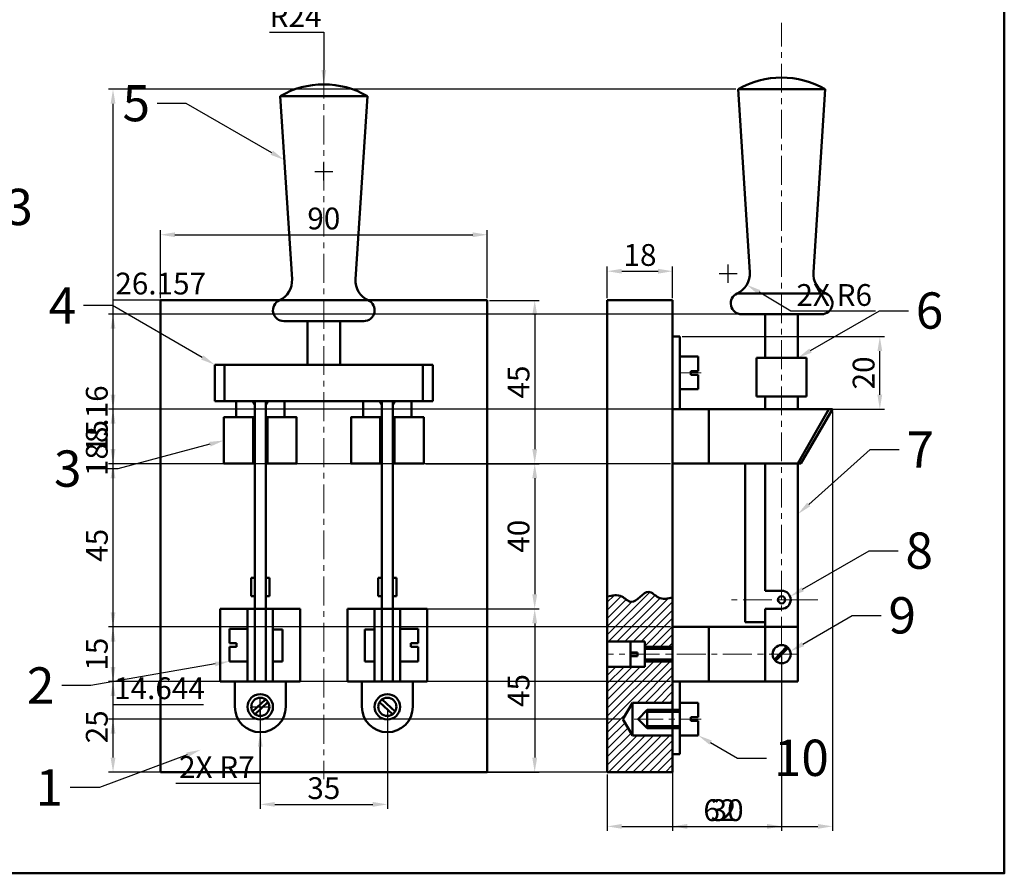
# Model space of a CAD drawing. Units: millimetres. Extents: x 1145 to 1687, y 12 to 400.
# Tile 5 of 6: x 1416 to 1687, y 12 to 247. Entities that reach past the tile are written whole.
import ezdxf
from ezdxf import colors
from ezdxf.entities.mleader import LeaderData, LeaderLine
from ezdxf.math import Vec2, Vec3

# ---------------------------------------------------------------- set-up
doc = ezdxf.new("R2010")
doc.units = ezdxf.units.MM
doc.header["$LTSCALE"] = 0.5
doc.linetypes.add('CENTER', pattern=[50.8, 31.75, -6.35, 6.35, -6.35])
for name, color, linetype, lineweight in [('M-CNTR', 1, 'CENTER', 18), ('M-DIMS', 2, 'Continuous', 25), ('M-HATC', 8, 'Continuous', 18), ('M-OUTL', 7, 'Continuous', 50), ('M-TEXT', 3, 'Continuous', 25)]:
    doc.layers.add(name, color=color, linetype=linetype, lineweight=lineweight)
doc.styles.get("Standard").update_dxf_attribs({"font": 'arial.ttf'})
doc.dimstyles.new('ISO-25', dxfattribs={"dimtxt": 6, "dimasz": 4, "dimexe": 1.25, "dimexo": 0.625, "dimtad": 1, "dimtoh": 1, "dimdec": 0, "dimtxsty": 'Standard', "dimcen": 2.5, "dimadec": 0, "dimazin": 0, "dimtfac": 1, "dimtdec": 0, "dimtofl": 0, "dimtmove": 0, "dimatfit": 3, "dimfxl": 1, "dimarcsym": 0})

# ---------------------------------------------------------------- blocks, each defined once
blk = doc.blocks.new('*D77')
at = {"layer": 'Defpoints', "color": 0, "ltscale": 0.5, "transparency": 16777216}
for p in [(1595.8, 178.16), (1577.8, 170.13), (1595.8, 170.13)]:
    blk.add_point(p, dxfattribs=at)
at = {"layer": 'M-DIMS', "color": 0, "lineweight": -2, "ltscale": 0.5, "transparency": 16777216}
for p, q in [((1577.8, 170.76), (1577.8, 179.41)), ((1595.8, 170.76), (1595.8, 179.41)), ((1581.8, 178.16), (1591.8, 178.16))]:
    blk.add_line(p, q, dxfattribs=at)
at = {"layer": 'M-DIMS', "color": 0, "ltscale": 0.5, "transparency": 16777216}
for points in [[(1581.8, 178.82), (1581.8, 177.49), (1577.8, 178.16)], [(1591.8, 178.82), (1591.8, 177.49), (1595.8, 178.16)]]:
    blk.add_solid(points, dxfattribs=at)
at = {"layer": 'M-DIMS', "color": 0, "ltscale": 0.5, "transparency": 16777216, "insert": (1586.8, 181.85), "char_height": 6, "attachment_point": 5}
blk.add_mtext('18', dxfattribs=at)
blk = doc.blocks.new('*D78')
at = {"layer": 'Defpoints', "color": 0, "ltscale": 0.5, "transparency": 16777216}
for p in [(1544.73, 188.21), (1454.73, 170.13), (1544.73, 170.13)]:
    blk.add_point(p, dxfattribs=at)
at = {"layer": 'M-DIMS', "color": 0, "lineweight": -2, "ltscale": 0.5, "transparency": 16777216}
for p, q in [((1454.73, 170.76), (1454.73, 189.46)), ((1458.73, 188.21), (1540.73, 188.21)), ((1544.73, 170.76), (1544.73, 189.46))]:
    blk.add_line(p, q, dxfattribs=at)
at = {"layer": 'M-DIMS', "color": 0, "ltscale": 0.5, "transparency": 16777216}
for points in [[(1458.73, 188.87), (1458.73, 187.54), (1454.73, 188.21)], [(1540.73, 188.87), (1540.73, 187.54), (1544.73, 188.21)]]:
    blk.add_solid(points, dxfattribs=at)
at = {"layer": 'M-DIMS', "color": 0, "ltscale": 0.5, "transparency": 16777216, "insert": (1499.73, 191.9), "char_height": 6, "attachment_point": 5}
blk.add_mtext('90', dxfattribs=at)
blk = doc.blocks.new('*D79')
at = {"layer": 'Defpoints', "color": 0, "ltscale": 0.5, "transparency": 16777216}
for p in [(1544.73, 170.13), (1527.23, 125.13), (1557.81, 125.13)]:
    blk.add_point(p, dxfattribs=at)
at = {"layer": 'M-DIMS', "color": 0, "lineweight": -2, "ltscale": 0.5, "transparency": 16777216}
for p, q in [((1545.36, 170.13), (1559.06, 170.13)), ((1557.81, 166.13), (1557.81, 129.13)), ((1527.86, 125.13), (1559.06, 125.13))]:
    blk.add_line(p, q, dxfattribs=at)
at = {"layer": 'M-DIMS', "color": 0, "ltscale": 0.5, "transparency": 16777216}
for points in [[(1557.14, 166.13), (1558.48, 166.13), (1557.81, 170.13)], [(1557.14, 129.13), (1558.48, 129.13), (1557.81, 125.13)]]:
    blk.add_solid(points, dxfattribs=at)
at = {"layer": 'M-DIMS', "color": 0, "ltscale": 0.5, "transparency": 16777216, "insert": (1554.13, 147.63), "char_height": 6, "attachment_point": 5, "rotation": 90}
blk.add_mtext('45', dxfattribs=at)
blk = doc.blocks.new('*D80')
at = {"layer": 'Defpoints', "color": 0, "ltscale": 0.5, "transparency": 16777216}
for p in [(1527.23, 125.13), (1527.23, 85.13), (1557.81, 85.13)]:
    blk.add_point(p, dxfattribs=at)
at = {"layer": 'M-DIMS', "color": 0, "lineweight": -2, "ltscale": 0.5, "transparency": 16777216}
for p, q in [((1527.86, 125.13), (1559.06, 125.13)), ((1557.81, 121.13), (1557.81, 89.13)), ((1527.86, 85.13), (1559.06, 85.13))]:
    blk.add_line(p, q, dxfattribs=at)
at = {"layer": 'M-DIMS', "color": 0, "ltscale": 0.5, "transparency": 16777216}
for points in [[(1557.14, 121.13), (1558.48, 121.13), (1557.81, 125.13)], [(1557.14, 89.13), (1558.48, 89.13), (1557.81, 85.13)]]:
    blk.add_solid(points, dxfattribs=at)
at = {"layer": 'M-DIMS', "color": 0, "ltscale": 0.5, "transparency": 16777216, "insert": (1554.12, 105.13), "char_height": 6, "attachment_point": 5, "rotation": 90}
blk.add_mtext('40', dxfattribs=at)
blk = doc.blocks.new('*D81')
at = {"layer": 'Defpoints', "color": 0, "ltscale": 0.5, "transparency": 16777216}
for p in [(1527.23, 85.13), (1527.23, 40.13), (1557.81, 40.13)]:
    blk.add_point(p, dxfattribs=at)
at = {"layer": 'M-DIMS', "color": 0, "lineweight": -2, "ltscale": 0.5, "transparency": 16777216}
for p, q in [((1527.86, 85.13), (1559.06, 85.13)), ((1557.81, 81.13), (1557.81, 44.13)), ((1527.86, 40.13), (1559.06, 40.13))]:
    blk.add_line(p, q, dxfattribs=at)
at = {"layer": 'M-DIMS', "color": 0, "ltscale": 0.5, "transparency": 16777216}
for points in [[(1557.14, 81.13), (1558.48, 81.13), (1557.81, 85.13)], [(1557.14, 44.13), (1558.48, 44.13), (1557.81, 40.13)]]:
    blk.add_solid(points, dxfattribs=at)
at = {"layer": 'M-DIMS', "color": 0, "ltscale": 0.5, "transparency": 16777216, "insert": (1554.13, 62.63), "char_height": 6, "attachment_point": 5, "rotation": 90}
blk.add_mtext('45', dxfattribs=at)
blk = doc.blocks.new('*D82')
at = {"layer": 'Defpoints', "color": 0, "ltscale": 0.5, "transparency": 16777216}
for p in [(1482.23, 58.13), (1517.23, 58.13), (1517.23, 31.26)]:
    blk.add_point(p, dxfattribs=at)
at = {"layer": 'M-DIMS', "color": 0, "lineweight": -2, "ltscale": 0.5, "transparency": 16777216}
for p, q in [((1482.23, 57.51), (1482.23, 30.01)), ((1517.23, 57.51), (1517.23, 30.01)), ((1486.23, 31.26), (1513.23, 31.26))]:
    blk.add_line(p, q, dxfattribs=at)
at = {"layer": 'M-DIMS', "color": 0, "ltscale": 0.5, "transparency": 16777216}
for points in [[(1486.23, 31.92), (1486.23, 30.59), (1482.23, 31.26)], [(1513.23, 31.92), (1513.23, 30.59), (1517.23, 31.26)]]:
    blk.add_solid(points, dxfattribs=at)
at = {"layer": 'M-DIMS', "color": 0, "ltscale": 0.5, "transparency": 16777216, "insert": (1499.73, 34.95), "char_height": 6, "attachment_point": 5}
blk.add_mtext('35', dxfattribs=at)
blk = doc.blocks.new('SCREW-HEAD')
at = {"ltscale": 0.5}
for p, q in [((0, 5), (4, 5)), ((0, 0), (0, 5)), ((4, 5), (4, 3)), ((4, 3), (5, 3)), ((5, 5), (5, 3)), ((5, 5), (9, 5)), ((9, 5), (9, 0)), ((9, 0), (0, 0))]:
    blk.add_line(p, q, dxfattribs=at)
blk = doc.blocks.new('HANDLE')
at = {"ltscale": 0.5}
for p, q in [((2, 62), (26, 62)), ((5.25, 11.58), (2, 62)), ((22.74, 11.58), (26, 62)), ((1.75, 5.73), (26.24, 5.73)), ((3, 0), (25, 0))]:
    blk.add_line(p, q, dxfattribs=at)
for centre, radius, start, end in [((14, 41.22), 24, 60, 120), ((-0.74, 11.19), 6, 294.5146, 3.6914), ((28.73, 11.19), 6, 176.3086, 245.4854), ((3, 3), 3, 114.5146, 270), ((25, 3), 3, 270, 65.4854)]:
    blk.add_arc(centre, radius, start, end, dxfattribs=at)
blk = doc.blocks.new('BRACKET')
at = {"ltscale": 0.5}
for p, q in [((15, 44), (0, 35.34)), ((15, 44), (15, 30)), ((0, 30), (0, 35.34)), ((0, 30), (0, 0)), ((15, 0), (15, 30)), ((35, 2), (15, 2)), ((35, 0), (35, 2)), ((0, 0), (15, 0)), ((15, 0), (35, 0))]:
    blk.add_line(p, q, dxfattribs=at)
blk = doc.blocks.new('TERMINAL-LUG-END')
at = {"ltscale": 0.5}
for p, q in [((0, 7), (0, 14)), ((14, 7), (14, 14))]:
    blk.add_line(p, q, dxfattribs=at)
blk.add_arc((7, 7), 7, 180, 0, dxfattribs=at)
blk = doc.blocks.new('TERMINAL-CLAMP')
at = {"ltscale": 0.5}
for p, q in [((0, 20), (0, 0)), ((0, 20), (22, 20)), ((22, 20), (22, 0)), ((0, 0), (22, 0))]:
    blk.add_line(p, q, dxfattribs=at)
blk = doc.blocks.new('*D102')
at = {"layer": 'Defpoints', "color": 0, "ltscale": 0.5, "transparency": 16777216}
for p in [(1441.68, 65.13), (1595.8, 65.13), (1595.8, 40.13)]:
    blk.add_point(p, dxfattribs=at)
at = {"layer": 'M-DIMS', "color": 0, "lineweight": -2, "ltscale": 0.5, "transparency": 16777216}
for p, q in [((1595.17, 65.13), (1440.43, 65.13)), ((1441.68, 44.13), (1441.68, 61.13)), ((1595.17, 40.13), (1440.43, 40.13))]:
    blk.add_line(p, q, dxfattribs=at)
at = {"layer": 'M-DIMS', "color": 0, "ltscale": 0.5, "transparency": 16777216}
for points in [[(1441.02, 61.13), (1442.35, 61.13), (1441.68, 65.13)], [(1441.02, 44.13), (1442.35, 44.13), (1441.68, 40.13)]]:
    blk.add_solid(points, dxfattribs=at)
at = {"layer": 'M-DIMS', "color": 0, "ltscale": 0.5, "transparency": 16777216, "insert": (1437.99, 52.63), "char_height": 6, "attachment_point": 5, "rotation": 90}
blk.add_mtext('25', dxfattribs=at)
blk = doc.blocks.new('*D103')
at = {"layer": 'Defpoints', "color": 0, "ltscale": 0.5, "transparency": 16777216}
for p in [(1441.68, 80.13), (1595.8, 80.13), (1595.8, 65.13)]:
    blk.add_point(p, dxfattribs=at)
at = {"layer": 'M-DIMS', "color": 0, "lineweight": -2, "ltscale": 0.5, "transparency": 16777216}
for p, q in [((1595.17, 80.13), (1440.43, 80.13)), ((1441.68, 69.13), (1441.68, 76.13)), ((1595.17, 65.13), (1440.43, 65.13))]:
    blk.add_line(p, q, dxfattribs=at)
at = {"layer": 'M-DIMS', "color": 0, "ltscale": 0.5, "transparency": 16777216}
for points in [[(1441.02, 76.13), (1442.35, 76.13), (1441.68, 80.13)], [(1441.02, 69.13), (1442.35, 69.13), (1441.68, 65.13)]]:
    blk.add_solid(points, dxfattribs=at)
at = {"layer": 'M-DIMS', "color": 0, "ltscale": 0.5, "transparency": 16777216, "insert": (1437.99, 72.63), "char_height": 6, "attachment_point": 5, "rotation": 90}
blk.add_mtext('15', dxfattribs=at)
blk = doc.blocks.new('*D104')
at = {"layer": 'Defpoints', "color": 0, "ltscale": 0.5, "transparency": 16777216}
for p in [(1441.68, 125.13), (1595.8, 125.13), (1595.8, 80.13)]:
    blk.add_point(p, dxfattribs=at)
at = {"layer": 'M-DIMS', "color": 0, "lineweight": -2, "ltscale": 0.5, "transparency": 16777216}
for p, q in [((1595.17, 125.13), (1440.43, 125.13)), ((1441.68, 84.13), (1441.68, 121.13)), ((1595.17, 80.13), (1440.43, 80.13))]:
    blk.add_line(p, q, dxfattribs=at)
at = {"layer": 'M-DIMS', "color": 0, "ltscale": 0.5, "transparency": 16777216}
for points in [[(1441.02, 121.13), (1442.35, 121.13), (1441.68, 125.13)], [(1441.02, 84.13), (1442.35, 84.13), (1441.68, 80.13)]]:
    blk.add_solid(points, dxfattribs=at)
at = {"layer": 'M-DIMS', "color": 0, "ltscale": 0.5, "transparency": 16777216, "insert": (1438.01, 102.63), "char_height": 6, "attachment_point": 5, "rotation": 90}
blk.add_mtext('45', dxfattribs=at)
blk = doc.blocks.new('*D105')
at = {"layer": 'Defpoints', "color": 0, "ltscale": 0.5, "transparency": 16777216}
for p in [(1441.68, 140.13), (1595.8, 140.13), (1595.8, 125.13)]:
    blk.add_point(p, dxfattribs=at)
at = {"layer": 'M-DIMS', "color": 0, "lineweight": -2, "ltscale": 0.5, "transparency": 16777216}
for p, q in [((1595.17, 140.13), (1440.43, 140.13)), ((1441.68, 129.13), (1441.68, 136.13)), ((1595.17, 125.13), (1440.43, 125.13))]:
    blk.add_line(p, q, dxfattribs=at)
at = {"layer": 'M-DIMS', "color": 0, "ltscale": 0.5, "transparency": 16777216}
for points in [[(1441.02, 136.13), (1442.35, 136.13), (1441.68, 140.13)], [(1441.02, 129.13), (1442.35, 129.13), (1441.68, 125.13)]]:
    blk.add_solid(points, dxfattribs=at)
at = {"layer": 'M-DIMS', "color": 0, "ltscale": 0.5, "transparency": 16777216, "insert": (1437.99, 132.63), "char_height": 6, "attachment_point": 5, "rotation": 90}
blk.add_mtext('15', dxfattribs=at)
blk = doc.blocks.new('*D106')
at = {"layer": 'Defpoints', "color": 0, "ltscale": 0.5, "transparency": 16777216}
for p in [(1639.8, 140.13), (1577.8, 40.13), (1639.8, 25.2)]:
    blk.add_point(p, dxfattribs=at)
at = {"layer": 'M-DIMS', "color": 0, "lineweight": -2, "ltscale": 0.5, "transparency": 16777216}
for p, q in [((1639.8, 139.51), (1639.8, 23.95)), ((1577.8, 39.51), (1577.8, 23.95)), ((1581.8, 25.2), (1635.8, 25.2))]:
    blk.add_line(p, q, dxfattribs=at)
at = {"layer": 'M-DIMS', "color": 0, "ltscale": 0.5, "transparency": 16777216}
for points in [[(1581.8, 25.86), (1581.8, 24.53), (1577.8, 25.2)], [(1635.8, 25.86), (1635.8, 24.53), (1639.8, 25.2)]]:
    blk.add_solid(points, dxfattribs=at)
at = {"layer": 'M-DIMS', "color": 0, "ltscale": 0.5, "transparency": 16777216, "insert": (1608.8, 28.89), "char_height": 6, "attachment_point": 5}
blk.add_mtext('62', dxfattribs=at)
blk = doc.blocks.new('*D107')
at = {"layer": 'Defpoints', "color": 0, "ltscale": 0.5, "transparency": 16777216}
for p in [(1441.68, 228.29), (1613.8, 228.29), (1577.8, 40.13)]:
    blk.add_point(p, dxfattribs=at)
at = {"layer": 'M-DIMS', "color": 0, "lineweight": -2, "ltscale": 0.5, "transparency": 16777216}
for p, q in [((1613.17, 228.29), (1440.43, 228.29)), ((1441.68, 44.13), (1441.68, 224.29)), ((1577.17, 40.13), (1440.43, 40.13))]:
    blk.add_line(p, q, dxfattribs=at)
at = {"layer": 'M-DIMS', "color": 0, "ltscale": 0.5, "transparency": 16777216}
for points in [[(1441.02, 224.29), (1442.35, 224.29), (1441.68, 228.29)], [(1441.02, 44.13), (1442.35, 44.13), (1441.68, 40.13)]]:
    blk.add_solid(points, dxfattribs=at)
at = {"layer": 'M-DIMS', "color": 0, "ltscale": 0.5, "transparency": 16777216, "insert": (1437.99, 134.21), "char_height": 6, "attachment_point": 5, "rotation": 90}
blk.add_mtext('188.16', dxfattribs=at)
blk = doc.blocks.new('*D108')
at = {"layer": 'Defpoints', "color": 0, "ltscale": 0.5, "transparency": 16777216}
for p in [(1595.8, 80.13), (1625.8, 72.63), (1625.8, 25.2)]:
    blk.add_point(p, dxfattribs=at)
at = {"layer": 'M-DIMS', "color": 0, "lineweight": -2, "ltscale": 0.5, "transparency": 16777216}
for p, q in [((1595.8, 79.51), (1595.8, 23.95)), ((1625.8, 72.01), (1625.8, 23.95)), ((1599.8, 25.2), (1621.8, 25.2))]:
    blk.add_line(p, q, dxfattribs=at)
at = {"layer": 'M-DIMS', "color": 0, "ltscale": 0.5, "transparency": 16777216}
for points in [[(1599.8, 25.86), (1599.8, 24.53), (1595.8, 25.2)], [(1621.8, 25.86), (1621.8, 24.53), (1625.8, 25.2)]]:
    blk.add_solid(points, dxfattribs=at)
at = {"layer": 'M-DIMS', "color": 0, "ltscale": 0.5, "transparency": 16777216, "insert": (1610.8, 28.89), "char_height": 6, "attachment_point": 5}
blk.add_mtext('30', dxfattribs=at)
blk = doc.blocks.new('*D109')
at = {"layer": 'Defpoints', "color": 0, "ltscale": 0.5, "transparency": 16777216}
for p in [(1441.68, 54.78), (1582.11, 54.78), (1577.8, 40.13)]:
    blk.add_point(p, dxfattribs=at)
at = {"layer": 'M-DIMS', "color": 0, "lineweight": -2, "ltscale": 0.5, "transparency": 16777216}
for p, q in [((1441.68, 54.78), (1441.68, 58.78)), ((1441.68, 58.78), (1466.63, 58.78)), ((1581.48, 54.78), (1440.43, 54.78)), ((1441.68, 44.13), (1441.68, 50.78)), ((1577.17, 40.13), (1440.43, 40.13))]:
    blk.add_line(p, q, dxfattribs=at)
at = {"layer": 'M-DIMS', "color": 0, "ltscale": 0.5, "transparency": 16777216}
for points in [[(1441.02, 50.78), (1442.35, 50.78), (1441.68, 54.78)], [(1441.02, 44.13), (1442.35, 44.13), (1441.68, 40.13)]]:
    blk.add_solid(points, dxfattribs=at)
at = {"layer": 'M-DIMS', "color": 0, "ltscale": 0.5, "transparency": 16777216, "insert": (1454.47, 62.47), "char_height": 6, "attachment_point": 5}
blk.add_mtext('14.644', dxfattribs=at)
blk = doc.blocks.new('*D110')
at = {"layer": 'Defpoints', "color": 0, "ltscale": 0.5, "transparency": 16777216}
for p in [(1441.68, 166.29), (1614.8, 166.29), (1621.3, 140.13)]:
    blk.add_point(p, dxfattribs=at)
at = {"layer": 'M-DIMS', "color": 0, "lineweight": -2, "ltscale": 0.5, "transparency": 16777216}
for p, q in [((1441.68, 166.29), (1441.68, 170.29)), ((1441.68, 170.29), (1467.32, 170.29)), ((1614.17, 166.29), (1440.43, 166.29)), ((1441.68, 144.13), (1441.68, 162.29)), ((1620.67, 140.13), (1440.43, 140.13))]:
    blk.add_line(p, q, dxfattribs=at)
at = {"layer": 'M-DIMS', "color": 0, "ltscale": 0.5, "transparency": 16777216}
for points in [[(1441.02, 162.29), (1442.35, 162.29), (1441.68, 166.29)], [(1441.02, 144.13), (1442.35, 144.13), (1441.68, 140.13)]]:
    blk.add_solid(points, dxfattribs=at)
at = {"layer": 'M-DIMS', "color": 0, "ltscale": 0.5, "transparency": 16777216, "insert": (1454.81, 173.98), "char_height": 6, "attachment_point": 5}
blk.add_mtext('26.157', dxfattribs=at)
blk = doc.blocks.new('*D111')
at = {"layer": 'Defpoints', "color": 0, "ltscale": 0.5, "transparency": 16777216}
for p in [(1597.8, 160.13), (1652.85, 160.13), (1595.8, 140.13)]:
    blk.add_point(p, dxfattribs=at)
at = {"layer": 'M-DIMS', "color": 0, "lineweight": -2, "ltscale": 0.5, "transparency": 16777216}
for p, q in [((1598.42, 160.13), (1654.1, 160.13)), ((1652.85, 144.13), (1652.85, 156.13)), ((1596.42, 140.13), (1654.1, 140.13))]:
    blk.add_line(p, q, dxfattribs=at)
at = {"layer": 'M-DIMS', "color": 0, "ltscale": 0.5, "transparency": 16777216}
for points in [[(1652.18, 156.13), (1653.51, 156.13), (1652.85, 160.13)], [(1652.18, 144.13), (1653.51, 144.13), (1652.85, 140.13)]]:
    blk.add_solid(points, dxfattribs=at)
at = {"layer": 'M-DIMS', "color": 0, "ltscale": 0.5, "transparency": 16777216, "insert": (1649.16, 150.13), "char_height": 6, "attachment_point": 5, "rotation": 90}
blk.add_mtext('20', dxfattribs=at)
blk = doc.blocks.new('*D119')
at = {"layer": 'Defpoints', "color": 0, "ltscale": 0.5, "transparency": 16777216}
for p in [(1499.73, 229.62), (1499.73, 205.62)]:
    blk.add_point(p, dxfattribs=at)
at = {"layer": 'M-DIMS', "color": 0, "lineweight": -2, "ltscale": 0.5, "transparency": 16777216}
for p, q in [((1484.79, 244.02), (1499.73, 244.02)), ((1499.73, 244.02), (1499.73, 233.62)), ((1499.73, 203.12), (1499.73, 208.12)), ((1497.23, 205.62), (1502.23, 205.62))]:
    blk.add_line(p, q, dxfattribs=at)
at = {"layer": 'M-DIMS', "color": 0, "ltscale": 0.5, "transparency": 16777216}
blk.add_solid([(1500.4, 233.62), (1499.07, 233.62), (1499.73, 229.62)], dxfattribs=at)
at = {"layer": 'M-DIMS', "color": 0, "ltscale": 0.5, "transparency": 16777216, "insert": (1491.95, 247.66), "char_height": 6, "attachment_point": 5}
blk.add_mtext('R24', dxfattribs=at)
blk = doc.blocks.new('*D120')
at = {"layer": 'Defpoints', "color": 0, "ltscale": 0.5, "transparency": 16777216}
for p in [(1482.23, 58.13), (1482.23, 51.13)]:
    blk.add_point(p, dxfattribs=at)
at = {"layer": 'M-DIMS', "color": 0, "lineweight": -2, "ltscale": 0.5, "transparency": 16777216}
for p, q in [((1482.23, 55.63), (1482.23, 60.63)), ((1479.73, 58.13), (1484.73, 58.13)), ((1482.23, 37.11), (1482.23, 47.13)), ((1458.94, 37.11), (1482.23, 37.11))]:
    blk.add_line(p, q, dxfattribs=at)
at = {"layer": 'M-DIMS', "color": 0, "ltscale": 0.5, "transparency": 16777216}
blk.add_solid([(1481.57, 47.13), (1482.9, 47.13), (1482.23, 51.13)], dxfattribs=at)
at = {"layer": 'M-DIMS', "color": 0, "ltscale": 0.5, "transparency": 16777216, "insert": (1470.27, 40.75), "char_height": 6, "attachment_point": 5}
blk.add_mtext('2X R7', dxfattribs=at)
blk = doc.blocks.new('*D121')
at = {"layer": 'Defpoints', "color": 0, "ltscale": 0.5, "transparency": 16777216}
for p in [(1611.06, 177.48), (1616.21, 174.4)]:
    blk.add_point(p, dxfattribs=at)
at = {"layer": 'M-DIMS', "color": 0, "lineweight": -2, "ltscale": 0.5, "transparency": 16777216}
for p, q in [((1611.06, 174.98), (1611.06, 179.98)), ((1608.56, 177.48), (1613.56, 177.48)), ((1628.33, 167.14), (1619.64, 172.34)), ((1651.63, 167.14), (1628.33, 167.14))]:
    blk.add_line(p, q, dxfattribs=at)
at = {"layer": 'M-DIMS', "color": 0, "ltscale": 0.5, "transparency": 16777216}
blk.add_solid([(1619.99, 172.92), (1619.3, 171.77), (1616.21, 174.4)], dxfattribs=at)
at = {"layer": 'M-DIMS', "color": 0, "ltscale": 0.5, "transparency": 16777216, "insert": (1640.29, 170.83), "char_height": 6, "attachment_point": 5}
blk.add_mtext('2X R6', dxfattribs=at)

msp = doc.modelspace()

# ---------------------------------------------------------------- hatches: boundary and pattern name
at = {"layer": 'M-HATC', "ltscale": 0.5}
h = msp.add_hatch(dxfattribs=at)
h.set_pattern_fill('ANSI31', color=256, scale=0.5)
h.set_pattern_definition([(45, (-479.3516, -223.5055), (-1.122532, 1.122532), [])])
edge = h.paths.add_edge_path()
edge.add_spline(control_points=[(1595.7981, 88.2598), (1594.455, 87.9688), (1592.0336, 87.444), (1588.5719, 91.6057), (1585.0835, 85.2802), (1581.6129, 89.3599), (1579.1872, 88.8247), (1577.7981, 88.5182)], knot_values=[0, 0, 0, 0, 3.87631709, 6.98846601, 12.57224805, 15.56070469, 19.56541111, 19.56541111, 19.56541111, 19.56541111], degree=3, periodic=0)
edge.add_line((1577.7981, 88.5182), (1577.7981, 76.1345))
edge.add_line((1577.7981, 76.1345), (1584.1572, 76.1345))
edge.add_line((1584.1572, 76.1345), (1588.1572, 76.1345))
edge.add_line((1588.1572, 76.1345), (1588.1572, 74.6345))
edge.add_line((1588.1572, 74.6345), (1595.7981, 74.6345))
edge.add_line((1595.7981, 74.6345), (1595.7981, 88.2598))
h.paths.add_polyline_path([(1588.1572, 69.1345), (1584.1572, 69.1345), (1577.7981, 69.1345), (1577.7981, 40.1345), (1595.7981, 40.1345), (1595.7981, 50.2788), (1584.7044, 50.2788), (1582.1063, 54.7788), (1584.7044, 59.2788), (1595.7981, 59.2788), (1595.7981, 70.6345), (1588.1572, 70.6345)])

# ---------------------------------------------------------------- linework, layer by layer
at = {"layer": 'M-CNTR', "ltscale": 0.5}
for p, q in [((1625.7981, 49.5797), (1625.7981, 246.6222)), ((1499.732, 233.7126), (1499.732, 38.2483)), ((1597.7981, 150.1345), (1603.6641, 150.1345)), ((1635.8068, 87.6345), (1611.1084, 87.6345)), ((1624.7981, 87.6345), (1629.3905, 87.6345)), ((1630.2981, 72.6345), (1577.7981, 72.6345)), ((1585.2422, 54.7788), (1603.6641, 54.7788))]:
    msp.add_line(p, q, dxfattribs=at)
at = {"layer": 'M-OUTL', "ltscale": 0.5}
for p, q in [((1611.7981, 172.2911), (1611.7981, 172.2911)), ((1544.732, 170.1345), (1454.732, 170.1345)), ((1454.732, 170.1345), (1454.732, 40.1345)), ((1485.732, 170.4049), (1485.732, 170.4049)), ((1544.732, 40.1345), (1544.732, 170.1345)), ((1577.7981, 170.1345), (1577.7981, 40.1345)), ((1595.7981, 170.1345), (1577.7981, 170.1345)), ((1595.7981, 40.1345), (1595.7981, 170.1345)), ((1621.2981, 166.2911), (1621.2981, 154.274)), ((1621.2981, 166.2911), (1630.2981, 166.2911)), ((1621.2981, 166.2911), (1630.2981, 166.2911)), ((1630.2981, 154.274), (1630.2981, 166.2911)), ((1495.232, 164.4049), (1495.232, 152.3878)), ((1495.232, 164.4049), (1504.232, 164.4049)), ((1495.232, 164.4049), (1504.232, 164.4049)), ((1504.232, 152.3878), (1504.232, 164.4049)), ((1499.732, 152.3878), (1469.732, 152.3878)), ((1469.732, 152.3878), (1469.732, 142.3878)), ((1472.422, 152.3878), (1472.422, 142.3878)), ((1504.232, 152.3878), (1495.232, 152.3878)), ((1529.732, 152.3878), (1504.232, 152.3878)), ((1527.042, 152.3878), (1527.042, 142.3878)), ((1529.732, 142.3878), (1529.732, 152.3878)), ((1630.2981, 154.274), (1618.907, 154.274)), ((1618.907, 154.274), (1618.907, 143.6345)), ((1630.2981, 154.274), (1632.6892, 154.274)), ((1632.6892, 154.274), (1632.6892, 143.6345)), ((1469.732, 142.3878), (1529.732, 142.3878)), ((1475.5773, 142.3878), (1475.5773, 137.9178)), ((1480.1771, 142.3878), (1480.732, 141.4746)), ((1480.732, 142.3878), (1480.732, 65.1345)), ((1483.732, 142.3878), (1483.732, 65.1345)), ((1484.2869, 142.3878), (1483.732, 141.4746)), ((1488.8867, 142.3878), (1488.8867, 137.9178)), ((1510.5773, 142.3878), (1510.5773, 137.9178)), ((1515.1771, 142.3878), (1515.732, 141.4746)), ((1515.732, 142.3878), (1515.732, 65.1345)), ((1518.732, 142.3878), (1518.732, 65.1345)), ((1519.2869, 142.3878), (1518.732, 141.4746)), ((1523.8867, 142.3878), (1523.8867, 137.9178)), ((1618.907, 143.6345), (1622.7981, 143.6345)), ((1621.2981, 140.1345), (1621.2981, 143.6345)), ((1622.7981, 143.6345), (1628.7981, 143.6345)), ((1632.6892, 143.6345), (1628.7981, 143.6345)), ((1630.2981, 140.1345), (1630.2981, 143.6345)), ((1605.7981, 125.1345), (1605.7981, 140.1345)), ((1638.832, 140.1345), (1630.2981, 125.1345)), ((1480.232, 137.9178), (1480.232, 125.1345)), ((1484.232, 137.9178), (1484.232, 125.1345)), ((1515.232, 137.9178), (1515.232, 125.1345)), ((1519.232, 137.9178), (1519.232, 125.1345)), ((1615.7981, 81.4343), (1615.7981, 125.1345)), ((1621.2981, 90.1345), (1621.2981, 125.1345)), ((1630.2981, 65.1345), (1630.2981, 125.1345)), ((1479.732, 88.6345), (1479.7244, 93.6345)), ((1479.7244, 93.6345), (1480.7244, 93.6345)), ((1484.7397, 93.6345), (1483.7397, 93.6345)), ((1484.732, 88.6345), (1484.7397, 93.6345)), ((1514.732, 88.6345), (1514.7244, 93.6345)), ((1514.7244, 93.6345), (1515.7244, 93.6345)), ((1519.7397, 93.6345), (1518.7397, 93.6345)), ((1519.732, 88.6345), (1519.7397, 93.6345)), ((1625.7981, 90.1345), (1621.2981, 90.1345)), ((1480.732, 88.6345), (1479.732, 88.6345)), ((1483.732, 88.6345), (1484.732, 88.6345)), ((1515.732, 88.6345), (1514.732, 88.6345)), ((1518.732, 88.6345), (1519.732, 88.6345)), ((1478.732, 85.1345), (1478.732, 65.1345)), ((1480.732, 85.1345), (1480.732, 65.1345)), ((1483.732, 85.1345), (1483.732, 65.1345)), ((1485.732, 85.1345), (1485.732, 65.1345)), ((1513.732, 85.1345), (1513.732, 65.1345)), ((1515.732, 85.1345), (1515.732, 65.1345)), ((1518.732, 85.1345), (1518.732, 65.1345)), ((1520.732, 85.1345), (1520.732, 65.1345)), ((1621.2981, 65.1345), (1621.2981, 85.1345)), ((1625.7981, 85.1345), (1621.2981, 85.1345)), ((1615.7981, 81.4343), (1621.2981, 81.4343)), ((1485.732, 79.4766), (1488.3976, 79.4766)), ((1488.3976, 79.4766), (1488.3976, 70.6345)), ((1513.732, 79.4766), (1511.0665, 79.4766)), ((1511.0665, 79.4766), (1511.0665, 70.6345)), ((1595.7981, 80.1345), (1595.7981, 65.1345)), ((1625.7981, 80.1345), (1595.7981, 80.1345)), ((1605.7981, 80.1345), (1605.7981, 65.1345)), ((1625.7981, 80.1345), (1630.2981, 80.1345)), ((1584.1572, 76.1345), (1577.7981, 76.1345)), ((1584.1572, 76.1345), (1584.1572, 69.1345)), ((1588.1572, 76.1345), (1584.1572, 76.1345)), ((1588.1572, 69.1345), (1588.1572, 76.1345)), ((1588.1572, 74.6345), (1595.7981, 74.6345)), ((1588.1572, 74.1345), (1595.7981, 74.1345)), ((1627.2281, 74.7247), (1623.7701, 71.1174)), ((1627.5891, 74.3787), (1624.1311, 70.7714)), ((1488.3976, 70.6345), (1485.732, 70.6345)), ((1511.0665, 70.6345), (1513.732, 70.6345)), ((1584.1572, 73.1345), (1586.1572, 73.1345)), ((1586.1572, 72.1345), (1584.1572, 72.1345)), ((1586.1572, 73.1345), (1586.1572, 72.1345)), ((1588.1572, 71.1345), (1595.7981, 71.1345)), ((1588.1572, 70.6345), (1595.7981, 70.6345)), ((1584.1572, 69.1345), (1577.7981, 69.1345)), ((1584.1572, 69.1345), (1588.1572, 69.1345)), ((1595.7981, 65.1345), (1625.7981, 65.1345)), ((1595.7981, 65.1345), (1595.7981, 45.1345)), ((1597.7981, 45.1345), (1597.7981, 65.1345)), ((1630.2981, 65.1345), (1621.2981, 65.1345)), ((1483.6776, 60.1742), (1480.1027, 56.8245)), ((1515.7865, 60.1742), (1519.3613, 56.8245)), ((1484.3613, 59.4445), (1480.7865, 56.0948)), ((1515.1027, 59.4445), (1518.6776, 56.0948)), ((1584.7044, 59.2788), (1582.1063, 54.7788)), ((1584.7044, 59.2788), (1584.7044, 50.2788)), ((1584.7044, 59.2788), (1595.7981, 59.2788)), ((1588.7981, 57.2788), (1586.2996, 54.7788)), ((1597.7981, 57.2788), (1588.7981, 57.2788)), ((1588.7981, 52.2788), (1588.7981, 57.2788)), ((1584.7044, 50.2788), (1582.1063, 54.7788)), ((1588.7981, 52.2788), (1586.2996, 54.7788)), ((1597.7981, 56.7788), (1588.7981, 56.7788)), ((1597.7981, 52.7788), (1588.7981, 52.7788)), ((1597.7981, 52.2788), (1588.7981, 52.2788)), ((1584.7044, 50.2788), (1595.7981, 50.2788)), ((1595.7981, 45.1345), (1597.7981, 45.1345)), ((1454.732, 40.1345), (1544.732, 40.1345)), ((1577.7981, 40.1345), (1595.7981, 40.1345))]:
    msp.add_line(p, q, dxfattribs=at)
msp.add_lwpolyline([(1145.3327, 400.1417), (1687.1285, 400.1417), (1687.1285, 12.2645), (1145.3327, 12.2645)], close=True, dxfattribs=at)
for points in [[(1480.732, 125.1345), (1472.232, 125.1345), (1472.232, 137.9178), (1480.732, 137.9178)], [(1483.732, 137.9178), (1492.232, 137.9178), (1492.232, 125.1345), (1483.732, 125.1345)], [(1515.732, 137.9178), (1507.232, 137.9178), (1507.232, 125.1345), (1515.732, 125.1345)], [(1518.732, 125.1345), (1527.232, 125.1345), (1527.232, 137.9178), (1518.732, 137.9178)]]:
    msp.add_lwpolyline(points, dxfattribs=at)
for centre, radius in [((1625.7981, 87.6345), 1), ((1625.7981, 87.6345), 1), ((1625.7981, 72.6345), 2.5), ((1625.7981, 72.6345), 2.5), ((1482.232, 58.1345), 3.5), ((1482.232, 58.1345), 2.5), ((1517.232, 58.1345), 3.5), ((1517.232, 58.1345), 2.5)]:
    msp.add_circle(centre, radius, dxfattribs=at)
msp.add_arc((1625.7981, 87.6345), 2.5, 270, 90, dxfattribs=at)
msp.add_open_spline([(1577.7981, 88.5182), (1579.1872, 88.8247), (1581.6129, 89.3599), (1585.0835, 85.2802), (1588.5719, 91.6057), (1592.0336, 87.444), (1594.455, 87.9688), (1595.7981, 88.2598)], degree=3, knots=[0, 0, 0, 0, 4.00470642, 6.99316306, 12.5769451, 15.68909402, 19.56541111, 19.56541111, 19.56541111, 19.56541111], dxfattribs=at)

# ---------------------------------------------------------------- block references
at = {"layer": 'M-OUTL'}
for name, p in [('HANDLE', (1485.7339, 164.4048)), ('HANDLE', (1611.8, 166.291)), ('TERMINAL-CLAMP', (1471.232, 65.134)), ('TERMINAL-CLAMP', (1506.232, 65.134)), ('TERMINAL-LUG-END', (1475.2324, 51.1344)), ('TERMINAL-LUG-END', (1510.2324, 51.1344))]:
    msp.add_blockref(name, p, dxfattribs=at)
at = {"layer": 'M-OUTL', "extrusion": (0, 0, -1), "zscale": -1, "rotation": 89.99999999999916}
msp.add_blockref('BRACKET', (-1595.7984, 125.1344), dxfattribs=at)
at = {"layer": 'M-OUTL'}
for p, rotation in [((1597.7983, 154.6349), 269.9999999999989), ((1478.7318, 70.634), 90.0000000000044), ((1520.7323, 79.6349), 269.9999999999964), ((1597.7983, 59.2792), 269.9999999999986)]:
    msp.add_blockref('SCREW-HEAD', p, dxfattribs=dict(at, rotation=rotation))

# ---------------------------------------------------------------- dimensions: what is measured, and where the dimension line sits
at = {"layer": 'M-DIMS', "ltscale": 0.5}
dim = msp.add_radius_dim(center=(1499.732, 205.6203), mpoint=(1499.732, 229.6203), dimstyle='ISO-25', override={"dimdec": 0, "dimlfac": 1, "dimrnd": 0, "dimzin": 0, "dimdsep": 46, "dimlunit": 2}, dxfattribs=at)
dim.commit()
dim.dimension.update_dxf_attribs({"geometry": '*D119', "text_midpoint": (1491.9508, 244.0203), "dimtype": 164})
for base, p1, p2, override, picture, middle in [((1441.682, 228.2911), (1577.7981, 40.1345), (1613.7981, 228.2911), {"dimdec": 2, "dimlfac": 1, "dimrnd": 0, "dimzin": 0, "dimdsep": 46, "dimlunit": 2}, '*D107', (1437.9936, 134.2128)), ((1441.682, 166.2911), (1621.2981, 140.1345), (1614.7981, 166.2911), {"dimdec": 3, "dimlfac": 1, "dimrnd": 0, "dimzin": 0, "dimdsep": 46, "dimlunit": 2}, '*D110', (1454.8125, 173.9795)), ((1557.811, 125.1345), (1544.732, 170.1345), (1527.232, 125.1345), {"dimclrd": 0, "dimclre": 0, "dimclrt": 0}, '*D79', (1554.1348, 147.6345)), ((1652.8481, 160.1345), (1595.7981, 140.1345), (1597.7981, 160.1345), {"dimdec": 0, "dimlfac": 1, "dimrnd": 0, "dimzin": 0, "dimdsep": 46, "dimlunit": 2}, '*D111', (1649.1596, 150.1345)), ((1441.682, 140.1345), (1595.7981, 125.1345), (1595.7981, 140.1345), {"dimdec": 0, "dimlfac": 1, "dimrnd": 0, "dimzin": 0, "dimdsep": 46, "dimlunit": 2}, '*D105', (1437.9936, 132.6345)), ((1441.682, 125.1345), (1595.7981, 80.1345), (1595.7981, 125.1345), {"dimdec": 0, "dimlfac": 1, "dimrnd": 0, "dimzin": 0, "dimdsep": 46, "dimlunit": 2}, '*D104', (1438.0059, 102.6345)), ((1557.811, 85.1345), (1527.232, 125.1345), (1527.232, 85.1345), {"dimclrd": 0, "dimclre": 0, "dimclrt": 0}, '*D80', (1554.1225, 105.1345)), ((1557.811, 40.1345), (1527.232, 85.1345), (1527.232, 40.1345), {"dimclrd": 0, "dimclre": 0, "dimclrt": 0}, '*D81', (1554.1348, 62.6345)), ((1441.682, 80.1345), (1595.7981, 65.1345), (1595.7981, 80.1345), {"dimdec": 0, "dimlfac": 1, "dimrnd": 0, "dimzin": 0, "dimdsep": 46, "dimlunit": 2}, '*D103', (1437.9936, 72.6345)), ((1441.682, 65.1345), (1595.7981, 40.1345), (1595.7981, 65.1345), {"dimdec": 0, "dimlfac": 1, "dimrnd": 0, "dimzin": 0, "dimdsep": 46, "dimlunit": 2}, '*D102', (1437.9936, 52.6345)), ((1441.682, 54.7788), (1577.7981, 40.1345), (1582.1063, 54.7788), {"dimdec": 3, "dimlfac": 1, "dimrnd": 0, "dimzin": 0, "dimdsep": 46, "dimlunit": 2}, '*D109', (1454.4666, 62.4672))]:
    dim = msp.add_linear_dim(base=base, p1=p1, p2=p2, angle=90, dimstyle='ISO-25', override=override, dxfattribs=at)
    dim.commit()
    dim.dimension.update_dxf_attribs({"geometry": picture, "text_midpoint": middle})
for base, p1, p2, override, picture, middle in [((1544.732, 188.2072), (1454.732, 170.1345), (1544.732, 170.1345), {"dimclrd": 0, "dimclre": 0, "dimclrt": 0}, '*D78', (1499.732, 191.8957)), ((1595.7981, 178.1569), (1577.7981, 170.1345), (1595.7981, 170.1345), {"dimclrd": 0, "dimclre": 0, "dimclrt": 0}, '*D77', (1586.7981, 181.8454)), ((1639.7981, 25.1983), (1577.7981, 40.1345), (1639.7981, 140.1345), {"dimdec": 0, "dimlfac": 1, "dimrnd": 0, "dimzin": 0, "dimdsep": 46, "dimlunit": 2}, '*D106', (1608.7981, 28.8867)), ((1625.7981, 25.1983), (1595.7981, 80.1345), (1625.7981, 72.6345), {"dimdec": 0, "dimlfac": 1, "dimrnd": 0, "dimzin": 0, "dimdsep": 46, "dimlunit": 2}, '*D108', (1610.7981, 28.8887)), ((1517.232, 31.2559), (1482.232, 58.1345), (1517.232, 58.1345), {"dimclrd": 0, "dimclre": 0, "dimclrt": 0}, '*D82', (1499.732, 34.9464))]:
    dim = msp.add_linear_dim(base=base, p1=p1, p2=p2, dimstyle='ISO-25', override=override, dxfattribs=at)
    dim.commit()
    dim.dimension.update_dxf_attribs({"geometry": picture, "text_midpoint": middle})
for center, mpoint, picture, middle in [((1611.0638, 177.4798), (1616.2123, 174.3988), '*D121', (1640.2923, 170.8331)), ((1482.232, 58.1345), (1482.232, 51.1345), '*D120', (1470.272, 40.7451))]:
    dim = msp.add_radius_dim(center=center, mpoint=mpoint, text='2X <>', dimstyle='ISO-25', override={"dimdec": 0, "dimlfac": 1, "dimrnd": 0, "dimzin": 0, "dimdsep": 46, "dimlunit": 2}, dxfattribs=at)
    dim.commit()
    dim.dimension.update_dxf_attribs({"geometry": picture, "text_midpoint": middle})

# ---------------------------------------------------------------- leaders
at = {"layer": 'M-TEXT', "ltscale": 0.5}
ml = msp.add_multileader_mtext('Standard', dxfattribs=at)
ml.set_content('5', color=256)
ml.set_leader_properties()
ml.build(insert=Vec2(0, 0))
ctx = ml.context
ctx.base_point, ctx.char_height, ctx.plane_origin = Vec3(1443.2349, 224.3889), 10, Vec3(1488.8679, 208.7989)
ctx.text_align_type = 2
notes = []
notes.append((ctx, [(0, (1, 1, 0), (1461.8652, 224.3889), (-1, 0), 8, [(0, [(1488.8679, 208.7989)], 0, [])])]))
ctx.mtext.insert, ctx.mtext.alignment, ctx.mtext.flow_direction = Vec3(1451.8652, 229.4742), 3, 5
ml = msp.add_multileader_mtext('Standard', dxfattribs=at)
ml.set_content('3', color=256)
ml.set_leader_properties()
ml.build(insert=Vec2(0, 0))
ctx = ml.context
ctx.base_point, ctx.char_height, ctx.plane_origin = Vec3(1410.0231, 195.7757), 10, Vec3(1379.2377, 156.3102)
notes.append((ctx, [(0, (1, 1, 0), (1402.0231, 195.7757), (1, 0), 8, [(0, [(1374.0331, 180.3937)], 0, [])])]))
ctx.mtext.insert, ctx.mtext.flow_direction = Vec3(1412.0231, 200.8644), 5
ml = msp.add_multileader_mtext('Standard', dxfattribs=at)
ml.set_content('4', color=256)
ml.set_leader_properties()
ml.build(insert=Vec2(0, 0))
ctx = ml.context
ctx.base_point, ctx.char_height, ctx.plane_origin = Vec3(1422.6066, 168.6741), 10, Vec3(1469.732, 152.3878)
ctx.text_align_type = 2
notes.append((ctx, [(0, (1, 1, 0), (1441.5234, 168.6741), (-1, 0), 8, [(0, [(1469.732, 152.3878)], 0, [])])]))
ctx.mtext.insert, ctx.mtext.alignment, ctx.mtext.flow_direction = Vec3(1431.5234, 173.6741), 3, 5
ml = msp.add_multileader_mtext('Standard', dxfattribs=at)
ml.set_content('6', color=256)
ml.set_leader_properties()
ml.build(insert=Vec2(0, 0))
ctx = ml.context
ctx.base_point, ctx.char_height, ctx.plane_origin = Vec3(1660.7528, 167.2383), 10, Vec3(1630.2981, 154.274)
notes.append((ctx, [(0, (1, 1, 0), (1652.7528, 167.2383), (1, 0), 8, [(0, [(1630.2981, 154.274)], 0, [])])]))
ctx.mtext.insert, ctx.mtext.flow_direction = Vec3(1662.7528, 172.3235), 5
ml = msp.add_multileader_mtext('Standard', dxfattribs=at)
ml.set_content('7', color=256)
ml.set_leader_properties()
ml.build(insert=Vec2(0, 0))
ctx = ml.context
ctx.base_point, ctx.char_height, ctx.plane_origin = Vec3(1658.2144, 129.0382), 10, Vec3(1630.2981, 111.2441)
notes.append((ctx, [(0, (1, 1, 0), (1650.2144, 129.0382), (1, 0), 8, [(0, [(1630.2981, 111.2441)], 0, [])])]))
ctx.mtext.insert, ctx.mtext.flow_direction = Vec3(1660.2144, 134.0382), 5
ml = msp.add_multileader_mtext('Standard', dxfattribs=at)
ml.set_content('3', color=256)
ml.set_leader_properties()
ml.build(insert=Vec2(0, 0))
ctx = ml.context
ctx.base_point, ctx.char_height, ctx.plane_origin = Vec3(1424.4421, 123.6926), 10, Vec3(1472.232, 131.5261)
ctx.text_align_type = 2
notes.append((ctx, [(0, (1, 1, 0), (1442.9906, 123.6926), (-1, 0), 8, [(0, [(1472.232, 131.5261)], 0, [])])]))
ctx.mtext.insert, ctx.mtext.alignment, ctx.mtext.flow_direction = Vec3(1432.9906, 128.7813), 3, 5
ml = msp.add_multileader_mtext('Standard', dxfattribs=at)
ml.set_content('8', color=256)
ml.set_leader_properties()
ml.build(insert=Vec2(0, 0))
ctx = ml.context
ctx.base_point, ctx.char_height, ctx.plane_origin = Vec3(1657.9073, 101.0942), 10, Vec3(1628.1346, 88.5237)
notes.append((ctx, [(0, (1, 1, 0), (1649.9073, 101.0942), (1, 0), 8, [(0, [(1628.1346, 88.5237)], 0, [])])]))
ctx.mtext.insert, ctx.mtext.flow_direction = Vec3(1659.9073, 106.1794), 5
ml = msp.add_multileader_mtext('Standard', dxfattribs=at)
ml.set_content('9', color=256)
ml.set_leader_properties()
ml.build(insert=Vec2(0, 0))
ctx = ml.context
ctx.base_point, ctx.char_height, ctx.plane_origin = Vec3(1653.2348, 83.259), 10, Vec3(1628.1749, 73.4094)
notes.append((ctx, [(0, (1, 1, 0), (1645.2348, 83.259), (1, 0), 8, [(0, [(1628.1749, 73.4094)], 0, [])])]))
ctx.mtext.insert, ctx.mtext.flow_direction = Vec3(1655.2348, 88.3442), 5
ml = msp.add_multileader_mtext('Standard', dxfattribs=at)
ml.set_content('2', color=256)
ml.set_leader_properties()
ml.build(insert=Vec2(0, 0))
ctx = ml.context
ctx.base_point, ctx.char_height, ctx.plane_origin = Vec3(1416.9179, 64.0153), 10, Vec3(1473.732, 70.6345)
ctx.text_align_type = 2
notes.append((ctx, [(0, (1, 1, 0), (1435.5413, 64.0153), (-1, 0), 8, [(0, [(1473.732, 70.6345)], 0, [])])]))
ctx.mtext.insert, ctx.mtext.alignment, ctx.mtext.flow_direction = Vec3(1425.5413, 69.0153), 3, 5
ml = msp.add_multileader_mtext('Standard', dxfattribs=at)
ml.set_content('10', color=256)
ml.set_leader_properties()
ml.build(insert=Vec2(0, 0))
ctx = ml.context
ctx.base_point, ctx.char_height, ctx.plane_origin = Vec3(1621.6638, 44.0055), 10, Vec3(1602.7981, 50.2788)
notes.append((ctx, [(0, (1, 1, 0), (1613.6638, 44.0055), (1, 0), 8, [(0, [(1602.7981, 50.2788)], 0, [])])]))
ctx.mtext.insert, ctx.mtext.flow_direction = Vec3(1623.6638, 49.0907), 5
ml = msp.add_multileader_mtext('Standard', dxfattribs=at)
ml.set_content('1', color=256)
ml.set_leader_properties()
ml.build(insert=Vec2(0, 0))
ctx = ml.context
ctx.base_point, ctx.char_height, ctx.plane_origin = Vec3(1422.2346, 35.9223), 10, Vec3(1465.8051, 46.302)
ctx.text_align_type = 2
notes.append((ctx, [(0, (1, 1, 0), (1437.9181, 35.9223), (-1, 0), 8, [(0, [(1465.8051, 46.302)], 0, [])])]))
ctx.mtext.insert, ctx.mtext.alignment, ctx.mtext.flow_direction = Vec3(1427.9181, 40.9223), 3, 5
for ctx, leaders in notes:
    for number, flags, end, landing, length, lines in leaders:
        leader = LeaderData()
        leader.index, (leader.has_last_leader_line, leader.has_dogleg_vector, leader.attachment_direction) = number, flags
        leader.last_leader_point, leader.dogleg_vector, leader.dogleg_length = Vec3(end), Vec3(landing), length
        for number, points, colour, breaks in lines:
            line = LeaderLine()
            line.index, line.vertices, line.color, line.breaks = number, Vec3.list(points), colors.encode_raw_color(colour), breaks
            leader.lines.append(line)
        ctx.leaders.append(leader)

doc.saveas('drawing.dxf')
